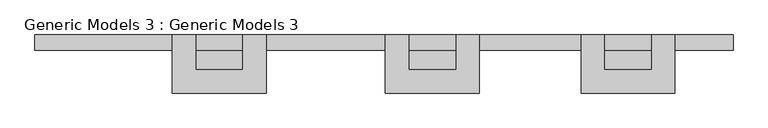
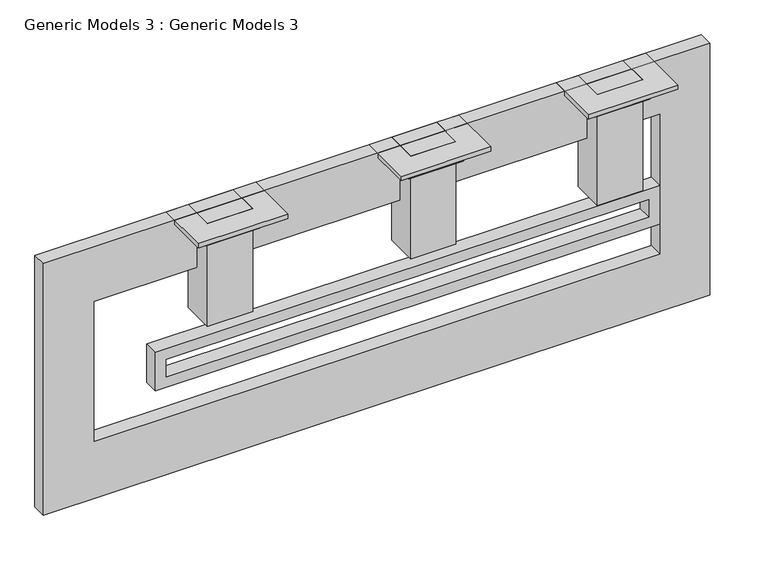
"""IFC4 building model written with IfcOpenShell, lengths in millimetres: proxy geometry, Generic Models 3 : Generic Models 3."""

from ifc_helpers import new_model, si_unit, frame, origin, place, context, project, spatial, polyline, circle_curve, ellipse_curve, outline, extrude, source, transform, mapped, element, save
from ifc_brep_helpers import plane_surface, cylinder_surface, advanced_brep


def generic_models_3_generic_models_3_686a9f3b(model_context):
    return source(origin(), model_context, "Body", "SolidModel", [
        extrude(outline(polyline([(0.0, 17876.4362453), (0.0, 14409.5114088), (-279.3976439, 14409.5114088), (-279.3976439, 17876.4362453), (0.0, 17876.4362453)]), holes=[polyline([(-76.2, 17800.2362453), (-203.1976439, 17800.2362453), (-203.1976439, 14485.7114088), (-76.2, 14485.7114088), (-76.2, 17800.2362453)])]), frame((0.0, -10122.9758122, 0.0), z_axis=(0.0, 1.0, 0.0), x_axis=(0.0, 0.0, 1.0)), (0.0, 0.0, 1.0), 101.6),
        advanced_brep(
        [(17836.0903184, -10021.3758122, 914.4), (17836.0903184, -10021.3758122, 882.65), (17778.3869392, -10021.3758122, 882.65), (17734.2127773, -10021.3758122, 832.946281), (17715.4403184, -10021.3758122, 780.5077263), (17683.6903184, -10021.3758122, 780.5077263), (17683.6903184, -10021.3758122, 914.4), (17836.0903184, -10402.3758122, 914.4), (17836.0903184, -10402.3758122, 882.65), (17221.2906872, -10402.3758122, 882.65), (17221.2906872, -10021.3758122, 882.65), (17278.9940664, -10021.3758122, 882.65), (17278.9940664, -10344.672433, 882.65), (17778.3869392, -10344.672433, 882.65), (17734.2127773, -10300.4982712, 832.946281), (17715.4403184, -10281.7258122, 780.5077263), (17341.9406872, -10281.7258122, 780.5077263), (17341.9406872, -10021.3758122, 780.5077263), (17373.6906872, -10021.3758122, 780.5077263), (17373.6906872, -10249.9758122, 780.5077263), (17683.6903184, -10249.9758122, 780.5077263), (17683.6903184, -10249.9758122, 914.4), (17373.6906872, -10249.9758122, 914.4), (17373.6906872, -10021.3758122, 914.4), (17221.2906872, -10021.3758122, 914.4), (17221.2906872, -10402.3758122, 914.4), (17323.1682282, -10300.4982712, 832.946281), (17323.1682282, -10021.3758122, 832.946281)],
        [
            (0, 1),
            (1, 2),
            (2, 3, circle_curve(frame((17710.4973209, -10021.3758122, 898.5051286), z_axis=(0.0, 1.0, 0.0), x_axis=(1.0, 0.0, 0.0)), 69.7164641)),
            (3, 4),
            (4, 5),
            (5, 6),
            (6, 0),
            (0, 7),
            (7, 8),
            (8, 1),
            (8, 9),
            (9, 10),
            (10, 11),
            (11, 12),
            (12, 13),
            (13, 2),
            (13, 14, ellipse_curve(frame((17710.4973209, -10276.7828147, 898.5051286), z_axis=(0.7071067811865475, 0.7071067811865475, 0.0), x_axis=(-0.7071067811865474, 0.7071067811865476, 0.0)), 98.5939691, 69.7164641)),
            (14, 3),
            (14, 15),
            (15, 4),
            (15, 16),
            (16, 17),
            (17, 18),
            (18, 19),
            (19, 20),
            (20, 5),
            (20, 21),
            (21, 6),
            (21, 22),
            (22, 23),
            (23, 24),
            (24, 25),
            (25, 7),
            (25, 9),
            (12, 26, ellipse_curve(frame((17346.8836846, -10276.7828147, 898.5051286), z_axis=(0.7071067811865475, -0.7071067811865475, 0.0), x_axis=(0.7071067811865476, 0.7071067811865474, 0.0)), 98.5939691, 69.7164641)),
            (26, 14),
            (26, 16),
            (19, 22),
            (23, 18),
            (17, 27),
            (27, 11, circle_curve(frame((17346.8836846, -10021.3758122, 898.5051286), z_axis=(0.0, 1.0, 0.0), x_axis=(-1.0, 0.0, 0.0)), 69.7164641)),
            (10, 24),
            (27, 26),
        ],
        [
            plane_surface(frame((17683.6903184, -10021.3758122, 914.4), z_axis=(0.0, 1.0, 0.0), x_axis=(0.0, 0.0, 1.0))),
            plane_surface(frame((17836.0903184, -10021.3758122, 914.4), z_axis=(1.0, 0.0, 0.0), x_axis=(0.0, -1.0, 0.0))),
            plane_surface(frame((17836.0903184, -10021.3758122, 882.65), z_axis=(0.0, 0.0, -1.0), x_axis=(0.0, -1.0, 0.0))),
            cylinder_surface(frame((17710.4973209, -10021.3758122, 898.5051286), z_axis=(0.0, 1.0, 0.0), x_axis=(1.0, 0.0, 0.0)), 69.7164641),
            plane_surface(frame((17734.2127773, -10021.3758122, 832.946281), z_axis=(0.941489129894626, 0.0, -0.33704334779114103), x_axis=(0.0, -1.0, 0.0))),
            plane_surface(frame((17715.4403184, -10021.3758122, 780.5077263), z_axis=(0.0, 0.0, -1.0), x_axis=(0.0, -1.0, 0.0))),
            plane_surface(frame((17683.6903184, -10021.3758122, 780.5077263), z_axis=(-1.0, 0.0, 0.0), x_axis=(0.0, -1.0, 0.0))),
            plane_surface(frame((17683.6903184, -10021.3758122, 914.4), z_axis=(0.0, 0.0, 1.0), x_axis=(0.0, -1.0, 0.0))),
            plane_surface(frame((17836.0903184, -10402.3758122, 914.4), z_axis=(0.0, -1.0, 0.0), x_axis=(-1.0, 0.0, 0.0))),
            cylinder_surface(frame((17683.6903184, -10276.7828147, 898.5051286), z_axis=(1.0, 0.0, 0.0), x_axis=(0.0, -1.0, 0.0)), 69.7164641),
            plane_surface(frame((17734.2127773, -10300.4982712, 832.946281), z_axis=(0.0, -0.941489129894626, -0.33704334779114103), x_axis=(-1.0, 0.0, 0.0))),
            plane_surface(frame((17683.6903184, -10249.9758122, 780.5077263), z_axis=(0.0, 1.0, 0.0), x_axis=(-1.0, 0.0, 0.0))),
            plane_surface(frame((17373.6906872, -10021.3758122, 914.4), z_axis=(0.0, 1.0, 0.0), x_axis=(0.0, 0.0, 1.0))),
            plane_surface(frame((17221.2906872, -10402.3758122, 914.4), z_axis=(-1.0, 0.0, 0.0), x_axis=(0.0, 1.0, 0.0))),
            cylinder_surface(frame((17346.8836846, -10249.9758122, 898.5051286), z_axis=(0.0, -1.0, 0.0), x_axis=(-1.0, 0.0, 0.0)), 69.7164641),
            plane_surface(frame((17323.1682282, -10300.4982712, 832.946281), z_axis=(-0.941489129894626, 0.0, -0.33704334779114103), x_axis=(0.0, 1.0, 0.0))),
            plane_surface(frame((17373.6906872, -10249.9758122, 780.5077263), z_axis=(1.0, 0.0, 0.0), x_axis=(0.0, 1.0, 0.0))),
        ],
        [
            (0, [[1, 2, 3, 4, 5, 6, 7]]),
            (1, [[-1, 8, 9, 10]]),
            (2, [[-2, -10, 11, 12, 13, 14, 15, 16]]),
            (3, [[-3, -16, 17, 18]]),
            (4, [[-4, -18, 19, 20]]),
            (5, [[-5, -20, 21, 22, 23, 24, 25, 26]]),
            (6, [[-6, -26, 27, 28]]),
            (7, [[-7, -28, 29, 30, 31, 32, 33, -8]]),
            (8, [[-9, -33, 34, -11]]),
            (9, [[-17, -15, 35, 36]]),
            (10, [[-19, -36, 37, -21]]),
            (11, [[-27, -25, 38, -29]]),
            (12, [[-31, 39, -23, 40, 41, -13, 42]]),
            (13, [[-34, -32, -42, -12]]),
            (14, [[-35, -14, -41, 43]]),
            (15, [[-37, -43, -40, -22]]),
            (16, [[-38, -24, -39, -30]]),
        ],
    ),
        advanced_brep(
        [(16553.6912345, -10021.3758122, 914.4), (16553.6912345, -10021.3758122, 882.65), (16495.9878553, -10021.3758122, 882.65), (16451.8136934, -10021.3758122, 832.946281), (16433.0412345, -10021.3758122, 780.5077263), (16401.2912345, -10021.3758122, 780.5077263), (16401.2912345, -10021.3758122, 914.4), (16553.6912345, -10402.3758122, 914.4), (16553.6912345, -10402.3758122, 882.65), (15938.8916032, -10402.3758122, 882.65), (15938.8916032, -10021.3758122, 882.65), (15996.5949824, -10021.3758122, 882.65), (15996.5949824, -10344.672433, 882.65), (16495.9878553, -10344.672433, 882.65), (16451.8136934, -10300.4982712, 832.946281), (16433.0412345, -10281.7258122, 780.5077263), (16059.5416032, -10281.7258122, 780.5077263), (16059.5416032, -10021.3758122, 780.5077263), (16091.2916032, -10021.3758122, 780.5077263), (16091.2916032, -10249.9758122, 780.5077263), (16401.2912345, -10249.9758122, 780.5077263), (16401.2912345, -10249.9758122, 914.4), (16091.2916032, -10249.9758122, 914.4), (16091.2916032, -10021.3758122, 914.4), (15938.8916032, -10021.3758122, 914.4), (15938.8916032, -10402.3758122, 914.4), (16040.7691443, -10300.4982712, 832.946281), (16040.7691443, -10021.3758122, 832.946281)],
        [
            (0, 1),
            (1, 2),
            (2, 3, circle_curve(frame((16428.098237, -10021.3758122, 898.5051286), z_axis=(0.0, 1.0, 0.0), x_axis=(1.0, 0.0, 0.0)), 69.7164641)),
            (3, 4),
            (4, 5),
            (5, 6),
            (6, 0),
            (0, 7),
            (7, 8),
            (8, 1),
            (8, 9),
            (9, 10),
            (10, 11),
            (11, 12),
            (12, 13),
            (13, 2),
            (13, 14, ellipse_curve(frame((16428.098237, -10276.7828147, 898.5051286), z_axis=(0.7071067811865475, 0.7071067811865475, 0.0), x_axis=(-0.7071067811865474, 0.7071067811865476, 0.0)), 98.5939691, 69.7164641)),
            (14, 3),
            (14, 15),
            (15, 4),
            (15, 16),
            (16, 17),
            (17, 18),
            (18, 19),
            (19, 20),
            (20, 5),
            (20, 21),
            (21, 6),
            (21, 22),
            (22, 23),
            (23, 24),
            (24, 25),
            (25, 7),
            (25, 9),
            (12, 26, ellipse_curve(frame((16064.4846007, -10276.7828147, 898.5051286), z_axis=(0.7071067811865475, -0.7071067811865475, 0.0), x_axis=(0.7071067811865476, 0.7071067811865474, 0.0)), 98.5939691, 69.7164641)),
            (26, 14),
            (26, 16),
            (19, 22),
            (23, 18),
            (17, 27),
            (27, 11, circle_curve(frame((16064.4846007, -10021.3758122, 898.5051286), z_axis=(0.0, 1.0, 0.0), x_axis=(-1.0, 0.0, 0.0)), 69.7164641)),
            (10, 24),
            (27, 26),
        ],
        [
            plane_surface(frame((16401.2912345, -10021.3758122, 914.4), z_axis=(0.0, 1.0, 0.0), x_axis=(0.0, 0.0, 1.0))),
            plane_surface(frame((16553.6912345, -10021.3758122, 914.4), z_axis=(1.0, 0.0, 0.0), x_axis=(0.0, -1.0, 0.0))),
            plane_surface(frame((16553.6912345, -10021.3758122, 882.65), z_axis=(0.0, 0.0, -1.0), x_axis=(0.0, -1.0, 0.0))),
            cylinder_surface(frame((16428.098237, -10021.3758122, 898.5051286), z_axis=(0.0, 1.0, 0.0), x_axis=(1.0, 0.0, 0.0)), 69.7164641),
            plane_surface(frame((16451.8136934, -10021.3758122, 832.946281), z_axis=(0.941489129894626, 0.0, -0.33704334779114103), x_axis=(0.0, -1.0, 0.0))),
            plane_surface(frame((16433.0412345, -10021.3758122, 780.5077263), z_axis=(0.0, 0.0, -1.0), x_axis=(0.0, -1.0, 0.0))),
            plane_surface(frame((16401.2912345, -10021.3758122, 780.5077263), z_axis=(-1.0, 0.0, 0.0), x_axis=(0.0, -1.0, 0.0))),
            plane_surface(frame((16401.2912345, -10021.3758122, 914.4), z_axis=(0.0, 0.0, 1.0), x_axis=(0.0, -1.0, 0.0))),
            plane_surface(frame((16553.6912345, -10402.3758122, 914.4), z_axis=(0.0, -1.0, 0.0), x_axis=(-1.0, 0.0, 0.0))),
            cylinder_surface(frame((16401.2912345, -10276.7828147, 898.5051286), z_axis=(1.0, 0.0, 0.0), x_axis=(0.0, -1.0, 0.0)), 69.7164641),
            plane_surface(frame((16451.8136934, -10300.4982712, 832.946281), z_axis=(0.0, -0.941489129894626, -0.33704334779114103), x_axis=(-1.0, 0.0, 0.0))),
            plane_surface(frame((16401.2912345, -10249.9758122, 780.5077263), z_axis=(0.0, 1.0, 0.0), x_axis=(-1.0, 0.0, 0.0))),
            plane_surface(frame((16091.2916032, -10021.3758122, 914.4), z_axis=(0.0, 1.0, 0.0), x_axis=(0.0, 0.0, 1.0))),
            plane_surface(frame((15938.8916032, -10402.3758122, 914.4), z_axis=(-1.0, 0.0, 0.0), x_axis=(0.0, 1.0, 0.0))),
            cylinder_surface(frame((16064.4846007, -10249.9758122, 898.5051286), z_axis=(0.0, -1.0, 0.0), x_axis=(-1.0, 0.0, 0.0)), 69.7164641),
            plane_surface(frame((16040.7691443, -10300.4982712, 832.946281), z_axis=(-0.941489129894626, 0.0, -0.33704334779114103), x_axis=(0.0, 1.0, 0.0))),
            plane_surface(frame((16091.2916032, -10249.9758122, 780.5077263), z_axis=(1.0, 0.0, 0.0), x_axis=(0.0, 1.0, 0.0))),
        ],
        [
            (0, [[1, 2, 3, 4, 5, 6, 7]]),
            (1, [[-1, 8, 9, 10]]),
            (2, [[-2, -10, 11, 12, 13, 14, 15, 16]]),
            (3, [[-3, -16, 17, 18]]),
            (4, [[-4, -18, 19, 20]]),
            (5, [[-5, -20, 21, 22, 23, 24, 25, 26]]),
            (6, [[-6, -26, 27, 28]]),
            (7, [[-7, -28, 29, 30, 31, 32, 33, -8]]),
            (8, [[-9, -33, 34, -11]]),
            (9, [[-17, -15, 35, 36]]),
            (10, [[-19, -36, 37, -21]]),
            (11, [[-27, -25, 38, -29]]),
            (12, [[-31, 39, -23, 40, 41, -13, 42]]),
            (13, [[-34, -32, -42, -12]]),
            (14, [[-35, -14, -41, 43]]),
            (15, [[-37, -43, -40, -22]]),
            (16, [[-38, -24, -39, -30]]),
        ],
    ),
        advanced_brep(
        [(15156.6912345, -10021.3758122, 914.4), (15156.6912345, -10021.3758122, 882.65), (15098.9878553, -10021.3758122, 882.65), (15054.8136934, -10021.3758122, 832.946281), (15036.0412345, -10021.3758122, 780.5077263), (15004.2912345, -10021.3758122, 780.5077263), (15004.2912345, -10021.3758122, 914.4), (15156.6912345, -10402.3758122, 914.4), (15156.6912345, -10402.3758122, 882.65), (14541.8916032, -10402.3758122, 882.65), (14541.8916032, -10021.3758122, 882.65), (14599.5949824, -10021.3758122, 882.65), (14599.5949824, -10344.672433, 882.65), (15098.9878553, -10344.672433, 882.65), (15054.8136934, -10300.4982712, 832.946281), (15036.0412345, -10281.7258122, 780.5077263), (14662.5416032, -10281.7258122, 780.5077263), (14662.5416032, -10021.3758122, 780.5077263), (14694.2916032, -10021.3758122, 780.5077263), (14694.2916032, -10249.9758122, 780.5077263), (15004.2912345, -10249.9758122, 780.5077263), (15004.2912345, -10249.9758122, 914.4), (14694.2916032, -10249.9758122, 914.4), (14694.2916032, -10021.3758122, 914.4), (14541.8916032, -10021.3758122, 914.4), (14541.8916032, -10402.3758122, 914.4), (14643.7691443, -10300.4982712, 832.946281), (14643.7691443, -10021.3758122, 832.946281)],
        [
            (0, 1),
            (1, 2),
            (2, 3, circle_curve(frame((15031.098237, -10021.3758122, 898.5051286), z_axis=(0.0, 1.0, 0.0), x_axis=(1.0, 0.0, 0.0)), 69.7164641)),
            (3, 4),
            (4, 5),
            (5, 6),
            (6, 0),
            (0, 7),
            (7, 8),
            (8, 1),
            (8, 9),
            (9, 10),
            (10, 11),
            (11, 12),
            (12, 13),
            (13, 2),
            (13, 14, ellipse_curve(frame((15031.098237, -10276.7828147, 898.5051286), z_axis=(0.7071067811865475, 0.7071067811865475, 0.0), x_axis=(-0.7071067811865474, 0.7071067811865476, 0.0)), 98.5939691, 69.7164641)),
            (14, 3),
            (14, 15),
            (15, 4),
            (15, 16),
            (16, 17),
            (17, 18),
            (18, 19),
            (19, 20),
            (20, 5),
            (20, 21),
            (21, 6),
            (21, 22),
            (22, 23),
            (23, 24),
            (24, 25),
            (25, 7),
            (25, 9),
            (12, 26, ellipse_curve(frame((14667.4846007, -10276.7828147, 898.5051286), z_axis=(0.7071067811865475, -0.7071067811865475, 0.0), x_axis=(0.7071067811865476, 0.7071067811865474, 0.0)), 98.5939691, 69.7164641)),
            (26, 14),
            (26, 16),
            (19, 22),
            (23, 18),
            (17, 27),
            (27, 11, circle_curve(frame((14667.4846007, -10021.3758122, 898.5051286), z_axis=(0.0, 1.0, 0.0), x_axis=(-1.0, 0.0, 0.0)), 69.7164641)),
            (10, 24),
            (27, 26),
        ],
        [
            plane_surface(frame((15004.2912345, -10021.3758122, 914.4), z_axis=(0.0, 1.0, 0.0), x_axis=(0.0, 0.0, 1.0))),
            plane_surface(frame((15156.6912345, -10021.3758122, 914.4), z_axis=(1.0, 0.0, 0.0), x_axis=(0.0, -1.0, 0.0))),
            plane_surface(frame((15156.6912345, -10021.3758122, 882.65), z_axis=(0.0, 0.0, -1.0), x_axis=(0.0, -1.0, 0.0))),
            cylinder_surface(frame((15031.098237, -10021.3758122, 898.5051286), z_axis=(0.0, 1.0, 0.0), x_axis=(1.0, 0.0, 0.0)), 69.7164641),
            plane_surface(frame((15054.8136934, -10021.3758122, 832.946281), z_axis=(0.941489129894626, 0.0, -0.33704334779114103), x_axis=(0.0, -1.0, 0.0))),
            plane_surface(frame((15036.0412345, -10021.3758122, 780.5077263), z_axis=(0.0, 0.0, -1.0), x_axis=(0.0, -1.0, 0.0))),
            plane_surface(frame((15004.2912345, -10021.3758122, 780.5077263), z_axis=(-1.0, 0.0, 0.0), x_axis=(0.0, -1.0, 0.0))),
            plane_surface(frame((15004.2912345, -10021.3758122, 914.4), z_axis=(0.0, 0.0, 1.0), x_axis=(0.0, -1.0, 0.0))),
            plane_surface(frame((15156.6912345, -10402.3758122, 914.4), z_axis=(0.0, -1.0, 0.0), x_axis=(-1.0, 0.0, 0.0))),
            cylinder_surface(frame((15004.2912345, -10276.7828147, 898.5051286), z_axis=(1.0, 0.0, 0.0), x_axis=(0.0, -1.0, 0.0)), 69.7164641),
            plane_surface(frame((15054.8136934, -10300.4982712, 832.946281), z_axis=(0.0, -0.941489129894626, -0.33704334779114103), x_axis=(-1.0, 0.0, 0.0))),
            plane_surface(frame((15004.2912345, -10249.9758122, 780.5077263), z_axis=(0.0, 1.0, 0.0), x_axis=(-1.0, 0.0, 0.0))),
            plane_surface(frame((14694.2916032, -10021.3758122, 914.4), z_axis=(0.0, 1.0, 0.0), x_axis=(0.0, 0.0, 1.0))),
            plane_surface(frame((14541.8916032, -10402.3758122, 914.4), z_axis=(-1.0, 0.0, 0.0), x_axis=(0.0, 1.0, 0.0))),
            cylinder_surface(frame((14667.4846007, -10249.9758122, 898.5051286), z_axis=(0.0, -1.0, 0.0), x_axis=(-1.0, 0.0, 0.0)), 69.7164641),
            plane_surface(frame((14643.7691443, -10300.4982712, 832.946281), z_axis=(-0.941489129894626, 0.0, -0.33704334779114103), x_axis=(0.0, 1.0, 0.0))),
            plane_surface(frame((14694.2916032, -10249.9758122, 780.5077263), z_axis=(1.0, 0.0, 0.0), x_axis=(0.0, 1.0, 0.0))),
        ],
        [
            (0, [[1, 2, 3, 4, 5, 6, 7]]),
            (1, [[-1, 8, 9, 10]]),
            (2, [[-2, -10, 11, 12, 13, 14, 15, 16]]),
            (3, [[-3, -16, 17, 18]]),
            (4, [[-4, -18, 19, 20]]),
            (5, [[-5, -20, 21, 22, 23, 24, 25, 26]]),
            (6, [[-6, -26, 27, 28]]),
            (7, [[-7, -28, 29, 30, 31, 32, 33, -8]]),
            (8, [[-9, -33, 34, -11]]),
            (9, [[-17, -15, 35, 36]]),
            (10, [[-19, -36, 37, -21]]),
            (11, [[-27, -25, 38, -29]]),
            (12, [[-31, 39, -23, 40, 41, -13, 42]]),
            (13, [[-34, -32, -42, -12]]),
            (14, [[-35, -14, -41, 43]]),
            (15, [[-37, -43, -40, -22]]),
            (16, [[-38, -24, -39, -30]]),
        ],
    ),
        extrude(outline(polyline([(914.4, 18217.5782182), (914.4, 13640.8433417), (-914.4, 13640.8433417), (-914.4, 18217.5782182), (914.4, 18217.5782182)]), holes=[polyline([(518.259226, 17876.4362453), (-497.740774, 17876.4362453), (-497.740774, 13990.2362453), (518.259226, 13990.2362453), (518.259226, 17876.4362453)])]), frame((0.0, -10122.9758122, 0.0), z_axis=(0.0, 1.0, 0.0), x_axis=(0.0, 0.0, 1.0)), (0.0, 0.0, 1.0), 101.6),
        extrude(outline(polyline([(15004.2912345, -10249.9758122), (14694.2916032, -10249.9758122), (14694.2916032, -10021.3758122), (15004.2912345, -10021.3758122), (15004.2912345, -10249.9758122)])), frame((0.0, 0.0, 166.9415952), z_axis=(0.0, 0.0, 1.0), x_axis=(1.0, 0.0, 0.0)), (0.0, 0.0, 1.0), 747.4584048),
        extrude(outline(polyline([(16401.2912345, -10249.9758122), (16091.2916032, -10249.9758122), (16091.2916032, -10021.3758122), (16401.2912345, -10021.3758122), (16401.2912345, -10249.9758122)])), frame((0.0, 0.0, 166.9415952), z_axis=(0.0, 0.0, 1.0), x_axis=(1.0, 0.0, 0.0)), (0.0, 0.0, 1.0), 747.4584048),
        extrude(outline(polyline([(17683.6903184, -10249.9758122), (17373.6906872, -10249.9758122), (17373.6906872, -10021.3758122), (17683.6903184, -10021.3758122), (17683.6903184, -10249.9758122)])), frame((0.0, 0.0, 108.0929449), z_axis=(0.0, 0.0, 1.0), x_axis=(1.0, 0.0, 0.0)), (0.0, 0.0, 1.0), 806.3070551),
    ])


if __name__ == "__main__":
    model = new_model("IFC4")
    model_context = context("Model", 3, world=origin())
    ifc_project = project(units=[si_unit("LENGTHUNIT", "METRE", prefix="MILLI")], contexts=[model_context])
    site = spatial("IfcSite", under=ifc_project)
    building = spatial("IfcBuilding", under=site)
    placement = place(None, origin())
    generic_models_3_generic_models_3_shape = generic_models_3_generic_models_3_686a9f3b(model_context)
    element("IfcBuildingElementProxy", 1, Name="Generic Models 3 : Generic Models 3", ObjectType="Generic Models 3 : Generic Models 3", at=placement, inside=building, context=model_context, shape_type="MappedRepresentation", body=[
        mapped(generic_models_3_generic_models_3_shape, transform((0.0, 0.0, 0.0), x_axis=(1.0, 0.0, 0.0), y_axis=(0.0, 1.0, 0.0), z_axis=(0.0, 0.0, 1.0))),
    ])
    save(model, "model.ifc")
